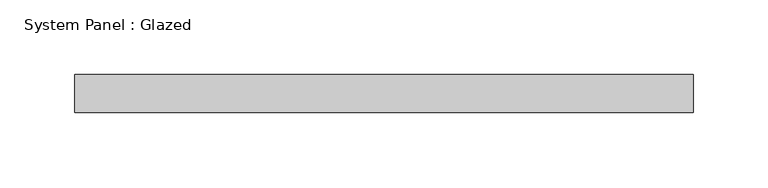
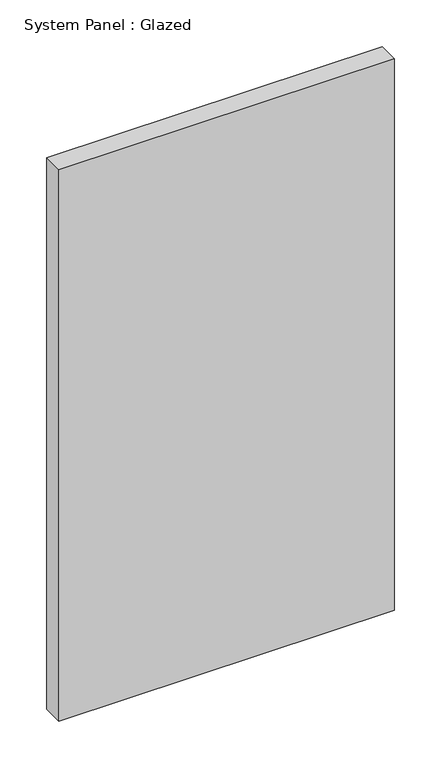
"""IFC4 building model written with IfcOpenShell, lengths in millimetres: plate geometry, System Panel : Glazed."""

from ifc_helpers import new_model, si_unit, origin, origin_with_axes, place, context, project, spatial, polyline, outline, extrude, source, transform, mapped, element, save


def system_panel_glazed_a6860354(model_context):
    return source(origin(), model_context, "Body", "SweptSolid", [
        extrude(outline(polyline([(206.375, 19.05), (-206.375, 19.05), (-206.375, 44.45), (206.375, 44.45), (206.375, 19.05)])), origin_with_axes(), (0.0, 0.0, 1.0), 717.55),
    ])


if __name__ == "__main__":
    model = new_model("IFC4")
    model_context = context("Model", 3, world=origin())
    ifc_project = project(units=[si_unit("LENGTHUNIT", "METRE", prefix="MILLI")], contexts=[model_context])
    site = spatial("IfcSite", under=ifc_project)
    building = spatial("IfcBuilding", under=site)
    placement = place(None, origin())
    system_panel_glazed_shape = system_panel_glazed_a6860354(model_context)
    element("IfcPlate", 1, ObjectType="System Panel : Glazed", at=placement, inside=building, context=model_context, shape_type="MappedRepresentation", body=[
        mapped(system_panel_glazed_shape, transform((0.0, 0.0, 0.0), x_axis=(1.0, 0.0, 0.0), y_axis=(0.0, 1.0, 0.0), z_axis=(0.0, 0.0, 1.0))),
    ])
    save(model, "model.ifc")

# Revit data of these elements
# Type "System Panel : Glazed"
#   Construction Type Id = "GSP4R"
#   Analytic Construction = "1/8 in Pilkington single glazing"
#   Visual Light Transmittance = 0.9
#   Solar Heat Gain Coefficient = 0.86
#   Heat Transfer Coefficient (U) = 1.18115 BTU/(h·ft²·°F)
#   Define Thermal Properties by = 1
# Element 1 (IfcPlate, "System Panel : Glazed")
#   Materials on its faces: "Glass"
# Materials
#   "Glass": class "Glass", colour RGB 0 128 192, transparency 0.75, Description = "Soda Lime Glass", Cost = 0
